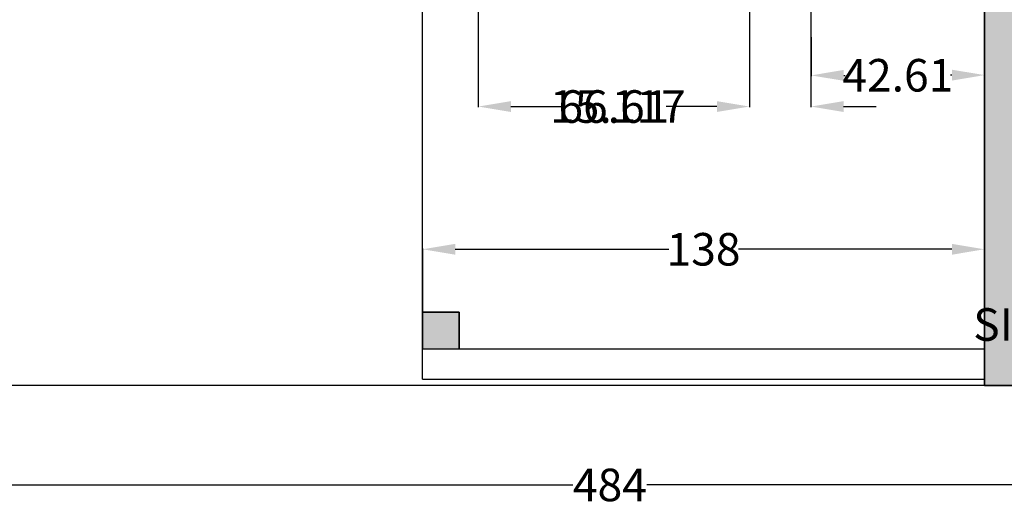
# Model space of a CAD drawing. Units: inches. Extents: x -52 to 678, y 23 to 685.
# Tile 2 of 11: x 189 to 431, y 23 to 143. Entities that reach past the tile are written whole.
import ezdxf

# ---------------------------------------------------------------- set-up
doc = ezdxf.new("R2010")
doc.units = ezdxf.units.IN
doc.header["$MEASUREMENT"] = 0
for name, color, linetype, lineweight in [('A-ANNO-DIMS', 2, 'Continuous', 18), ('A-COLS', 7, 'Continuous', 35), ('A-FLOR', 7, 'Continuous', 25), ('A-WALL', 7, 'Continuous', 35)]:
    doc.layers.add(name, color=color, linetype=linetype, lineweight=lineweight)
doc.layers.add('A-COLS-PATT', color=18, linetype='Continuous', lineweight=13, true_color=0x000000)
doc.layers.add('A-WALL-PATT', color=18, linetype='Continuous', lineweight=13, true_color=0x000000)
doc.styles.get("Standard").update_dxf_attribs({"font": 'arial.ttf'})
doc.dimstyles.get("Standard").update_dxf_attribs({"dimtxt": 8, "dimasz": 8, "dimexe": 0.18, "dimexo": 0.0625, "dimgap": 0.09, "dimtad": 0, "dimtih": 1, "dimtoh": 1, "dimdec": 0, "dimzin": 0, "dimdsep": 46, "dimlunit": 3, "dimtxsty": 'Standard', "dimcen": 0.09, "dimadec": 0, "dimazin": 0, "dimtfac": 1, "dimtdec": 0, "dimtofl": 0, "dimtmove": 0, "dimatfit": 3, "dimfxl": 1, "dimtolj": 1, "dimtzin": 0, "dimarcsym": 0})

# ---------------------------------------------------------------- blocks, each defined once
blk = doc.blocks.new('*D17')
at = {"layer": 'A-ANNO-DIMS', "color": 0, "lineweight": -2, "transparency": 16777216}
for p, q in [((471.9, 82.07), (471.9, 90.07)), ((470.17, 74.07), (472.08, 74.07)), ((470.17, 62.13), (472.08, 62.13)), ((471.9, 54.13), (471.9, 46.13))]:
    blk.add_line(p, q, dxfattribs=at)
at = {"layer": 'A-ANNO-DIMS', "color": 0, "transparency": 16777216}
for points in [[(470.56, 82.07), (473.23, 82.07), (471.9, 74.07)], [(470.56, 54.13), (473.23, 54.13), (471.9, 62.13)]]:
    blk.add_solid(points, dxfattribs=at)
at = {"layer": 'Defpoints', "color": 0, "transparency": 16777216}
for p in [(470.1, 74.07), (471.9, 74.07), (470.1, 62.13)]:
    blk.add_point(p, dxfattribs=at)
at = {"layer": 'A-ANNO-DIMS', "color": 0, "transparency": 16777216, "insert": (471.9, 68.1), "char_height": 8, "attachment_point": 5}
blk.add_mtext('\\A1;SIDE TABLE 12 TYP.', dxfattribs=at)
blk = doc.blocks.new('*D39')
at = {"layer": 'A-ANNO-DIMS', "color": 0, "lineweight": -2, "transparency": 16777216}
for p, q in [((91.61, 327.06), (91.61, 28.49)), ((575.61, 53.06), (575.61, 28.49)), ((99.61, 28.67), (324.53, 28.67)), ((567.61, 28.67), (342.68, 28.67))]:
    blk.add_line(p, q, dxfattribs=at)
at = {"layer": 'A-ANNO-DIMS', "color": 0, "transparency": 16777216}
for points in [[(99.61, 30), (99.61, 27.33), (91.61, 28.67)], [(567.61, 30), (567.61, 27.33), (575.61, 28.67)]]:
    blk.add_solid(points, dxfattribs=at)
at = {"layer": 'Defpoints', "color": 0, "transparency": 16777216}
for p in [(91.61, 327.13), (575.61, 53.13), (575.61, 28.67)]:
    blk.add_point(p, dxfattribs=at)
at = {"layer": 'A-ANNO-DIMS', "color": 0, "transparency": 16777216, "insert": (333.61, 28.67), "char_height": 8, "attachment_point": 5}
blk.add_mtext('\\A1;484', dxfattribs=at)
blk = doc.blocks.new('*D40')
at = {"layer": 'A-ANNO-DIMS', "color": 0, "lineweight": -2, "transparency": 16777216}
for p, q in [((358.67, 525.13), (600.25, 525.13)), ((600.07, 517.13), (600.07, 293.23)), ((600.07, 61.13), (600.07, 285.02)), ((575.67, 53.13), (600.25, 53.13))]:
    blk.add_line(p, q, dxfattribs=at)
at = {"layer": 'A-ANNO-DIMS', "color": 0, "transparency": 16777216}
for points in [[(598.73, 517.13), (601.4, 517.13), (600.07, 525.13)], [(598.73, 61.13), (601.4, 61.13), (600.07, 53.13)]]:
    blk.add_solid(points, dxfattribs=at)
at = {"layer": 'Defpoints', "color": 0, "transparency": 16777216}
for p in [(358.61, 525.13), (600.07, 525.13), (575.61, 53.13)]:
    blk.add_point(p, dxfattribs=at)
at = {"layer": 'A-ANNO-DIMS', "color": 0, "transparency": 16777216, "insert": (600.07, 289.13), "char_height": 8, "attachment_point": 5}
blk.add_mtext('\\A1;472', dxfattribs=at)
blk = doc.blocks.new('*D47')
at = {"layer": 'A-ANNO-DIMS', "color": 0, "lineweight": -2, "transparency": 16777216}
for p, q in [((188.54, 146.13), (66.97, 146.13)), ((67.15, 138.13), (67.15, 103.8)), ((67.15, 61.13), (67.15, 95.45)), ((425.54, 53.13), (66.97, 53.13))]:
    blk.add_line(p, q, dxfattribs=at)
at = {"layer": 'A-ANNO-DIMS', "color": 0, "transparency": 16777216}
for points in [[(65.81, 138.13), (68.48, 138.13), (67.15, 146.13)], [(65.81, 61.13), (68.48, 61.13), (67.15, 53.13)]]:
    blk.add_solid(points, dxfattribs=at)
at = {"layer": 'Defpoints', "color": 0, "transparency": 16777216}
for p in [(67.15, 146.13), (188.61, 146.13), (425.61, 53.13)]:
    blk.add_point(p, dxfattribs=at)
at = {"layer": 'A-ANNO-DIMS', "color": 0, "transparency": 16777216, "insert": (67.15, 99.63), "char_height": 8, "attachment_point": 5}
blk.add_mtext('\\A1;93', dxfattribs=at)
blk = doc.blocks.new('*D50')
at = {"layer": 'A-ANNO-DIMS', "color": 0, "lineweight": -2, "transparency": 16777216}
for p, q in [((287.61, 62.19), (287.61, 86.77)), ((295.61, 86.59), (348.05, 86.59)), ((417.61, 86.59), (365.16, 86.59)), ((425.61, 62.19), (425.61, 86.77))]:
    blk.add_line(p, q, dxfattribs=at)
at = {"layer": 'A-ANNO-DIMS', "color": 0, "transparency": 16777216}
for points in [[(295.61, 87.92), (295.61, 85.25), (287.61, 86.59)], [(417.61, 87.92), (417.61, 85.25), (425.61, 86.59)]]:
    blk.add_solid(points, dxfattribs=at)
at = {"layer": 'Defpoints', "color": 0, "transparency": 16777216}
for p in [(425.61, 86.59), (287.61, 62.13), (425.61, 62.13)]:
    blk.add_point(p, dxfattribs=at)
at = {"layer": 'A-ANNO-DIMS', "color": 0, "transparency": 16777216, "insert": (356.61, 86.59), "char_height": 8, "attachment_point": 5}
blk.add_mtext('\\A1;138', dxfattribs=at)
blk = doc.blocks.new('*D78')
at = {"layer": 'A-ANNO-DIMS', "color": 0, "lineweight": -2, "transparency": 16777216}
for p, q in [((301.27, 146.06), (301.27, 121.49)), ((367.88, 146.06), (367.88, 121.49)), ((309.27, 121.67), (321.74, 121.67)), ((359.88, 121.67), (347.41, 121.67))]:
    blk.add_line(p, q, dxfattribs=at)
at = {"layer": 'A-ANNO-DIMS', "color": 0, "transparency": 16777216}
for points in [[(309.27, 123), (309.27, 120.33), (301.27, 121.67)], [(359.88, 123), (359.88, 120.33), (367.88, 121.67)]]:
    blk.add_solid(points, dxfattribs=at)
at = {"layer": 'Defpoints', "color": 0, "transparency": 16777216}
for p in [(301.27, 146.13), (367.88, 146.13), (301.27, 121.67)]:
    blk.add_point(p, dxfattribs=at)
at = {"layer": 'A-ANNO-DIMS', "color": 0, "transparency": 16777216, "insert": (334.58, 121.67), "char_height": 8, "attachment_point": 5}
blk.add_mtext('\\A1;66.61', dxfattribs=at)
blk = doc.blocks.new('*D79')
at = {"layer": 'A-ANNO-DIMS', "color": 0, "lineweight": -2, "transparency": 16777216}
for p, q in [((383, 153.72), (383.04, 129.14)), ((425.61, 153.8), (425.65, 129.22)), ((391.04, 129.34), (391.37, 129.34)), ((417.65, 129.39), (417.32, 129.38))]:
    blk.add_line(p, q, dxfattribs=at)
at = {"layer": 'A-ANNO-DIMS', "color": 0, "transparency": 16777216}
for points in [[(391.04, 130.67), (391.05, 128), (383.04, 129.32)], [(417.65, 130.72), (417.65, 128.05), (425.65, 129.4)]]:
    blk.add_solid(points, dxfattribs=at)
at = {"layer": 'Defpoints', "color": 0, "transparency": 16777216}
for p in [(383, 153.78), (425.61, 153.86), (383.04, 129.32)]:
    blk.add_point(p, dxfattribs=at)
at = {"layer": 'A-ANNO-DIMS', "color": 0, "transparency": 16777216, "insert": (404.35, 129.36), "char_height": 8, "attachment_point": 5}
blk.add_mtext('\\A1;42.61', dxfattribs=at)
blk = doc.blocks.new('*D80')
at = {"layer": 'A-ANNO-DIMS', "color": 0, "lineweight": -2, "transparency": 16777216}
for p, q in [((367.88, 146.06), (367.88, 121.49)), ((383, 146.06), (383, 121.49)), ((359.88, 121.67), (351.88, 121.67)), ((391, 121.67), (399, 121.67))]:
    blk.add_line(p, q, dxfattribs=at)
at = {"layer": 'A-ANNO-DIMS', "color": 0, "transparency": 16777216}
for points in [[(359.88, 123), (359.88, 120.33), (367.88, 121.67)], [(391, 123), (391, 120.33), (383, 121.67)]]:
    blk.add_solid(points, dxfattribs=at)
at = {"layer": 'Defpoints', "color": 0, "transparency": 16777216}
for p in [(367.88, 146.13), (383, 146.13), (367.88, 121.67)]:
    blk.add_point(p, dxfattribs=at)
at = {"layer": 'A-ANNO-DIMS', "color": 0, "transparency": 16777216, "insert": (335.56, 121.67), "char_height": 8, "attachment_point": 5}
blk.add_mtext('\\A1;15.117', dxfattribs=at)

msp = doc.modelspace()

# ---------------------------------------------------------------- hatches: boundary and pattern name
at = {"layer": 'A-COLS-PATT'}
h = msp.add_hatch(color=256, dxfattribs=at)
h.dxf.hatch_style = 1
h.paths.add_polyline_path([(296.6053, 62.1267), (296.6053, 71.1267), (287.6053, 71.1267), (287.6053, 62.1267)])
at = {"layer": 'A-WALL-PATT'}
h = msp.add_hatch(color=256, dxfattribs=at)
h.dxf.hatch_style = 1
h.paths.add_polyline_path([(434.6053, 239.1267), (434.6053, 285.9421), (425.6053, 285.9421), (425.6053, 239.1267), (425.6053, 53.1267), (468.8253, 53.1267), (468.8253, 62.1267), (434.6053, 62.1267)])

# ---------------------------------------------------------------- linework, layer by layer
at = {"layer": 'A-COLS'}
for p, q in [((287.6053, 62.1267), (287.6053, 71.1267)), ((287.6053, 71.1267), (296.6053, 71.1267)), ((296.6053, 71.1267), (296.6053, 62.1267))]:
    msp.add_line(p, q, dxfattribs=at)
at = {"layer": 'A-FLOR'}
for p, q in [((287.6053, 54.6267), (287.6053, 146.1267)), ((287.6053, 62.1267), (425.6053, 62.1267)), ((287.6053, 62.1267), (425.6053, 62.1267)), ((287.6053, 54.6267), (425.6053, 54.6267))]:
    msp.add_line(p, q, dxfattribs=at)
at = {"layer": 'A-WALL'}
for p, q in [((425.6053, 53.1267), (425.6053, 239.1267)), ((425.6053, 53.1267), (425.6053, 66.1267)), ((425.6053, 53.1267), (468.8253, 53.1267)), ((468.8253, 53.1267), (425.6053, 53.1267))]:
    msp.add_line(p, q, dxfattribs=at)

# ---------------------------------------------------------------- dimensions: what is measured, and where the dimension line sits
at = {"layer": 'A-ANNO-DIMS'}
for base, p1, p2, angle, override, picture, middle in [((600.0653, 525.1267), (575.6053, 53.1267), (358.6053, 525.1267), 90, {"dimdec": 0, "dimlfac": 1, "dimrnd": 0, "dimzin": 0, "dimdsep": 46, "dimlunit": 2}, '*D40', (600.0653, 289.1267)), ((383.0434, 129.3224), (425.6053, 153.86), (382.9989, 153.7824), 180.104418, {"dimdec": 2, "dimlfac": 1, "dimrnd": 0, "dimzin": 0, "dimdsep": 46, "dimlunit": 2}, '*D79', (404.3466, 129.3613)), ((67.1453, 146.1267), (425.6053, 53.1267), (188.6053, 146.1267), 90, {"dimdec": 0, "dimlfac": 1, "dimrnd": 0, "dimzin": 0, "dimdsep": 46, "dimlunit": 2}, '*D47', (67.1453, 99.6267)), ((301.2728, 121.6667), (367.8819, 146.1267), (301.2728, 146.1267), 180, {"dimdec": 2, "dimlfac": 1, "dimrnd": 0, "dimzin": 0, "dimdsep": 46, "dimlunit": 2}, '*D78', (334.5773, 121.6667)), ((367.8819, 121.6667), (382.9989, 146.1267), (367.8819, 146.1267), 180, {"dimdec": 3, "dimlfac": 1, "dimrnd": 0, "dimzin": 0, "dimdsep": 46, "dimlunit": 2}, '*D80', (335.5627, 121.6667))]:
    dim = msp.add_linear_dim(base=base, p1=p1, p2=p2, angle=angle, dimstyle='Standard', override=override, dxfattribs=at)
    dim.commit()
    dim.dimension.update_dxf_attribs({"geometry": picture, "text_midpoint": middle})
for base, p1, p2, picture, middle in [((575.6053, 28.6667), (91.6053, 327.1267), (575.6053, 53.1267), '*D39', (333.6053, 28.6667)), ((425.6053, 86.5867), (287.6053, 62.1267), (425.6053, 62.1267), '*D50', (356.6053, 86.5867))]:
    dim = msp.add_linear_dim(base=base, p1=p1, p2=p2, dimstyle='Standard', override={"dimdec": 0, "dimlfac": 1, "dimrnd": 0, "dimzin": 0, "dimdsep": 46, "dimlunit": 2}, dxfattribs=at)
    dim.commit()
    dim.dimension.update_dxf_attribs({"geometry": picture, "text_midpoint": middle})
dim = msp.add_linear_dim(base=(471.896, 74.0746), p1=(470.1039, 62.1267), p2=(470.1039, 74.0746), angle=90, text='SIDE TABLE <> TYP.', dimstyle='Standard', override={"dimdec": 0, "dimlfac": 1, "dimrnd": 0, "dimzin": 0, "dimdsep": 46, "dimlunit": 2}, dxfattribs=at)
dim.commit()
dim.dimension.update_dxf_attribs({"geometry": '*D17', "text_midpoint": (471.896, 68.1007)})

doc.saveas('drawing.dxf')
